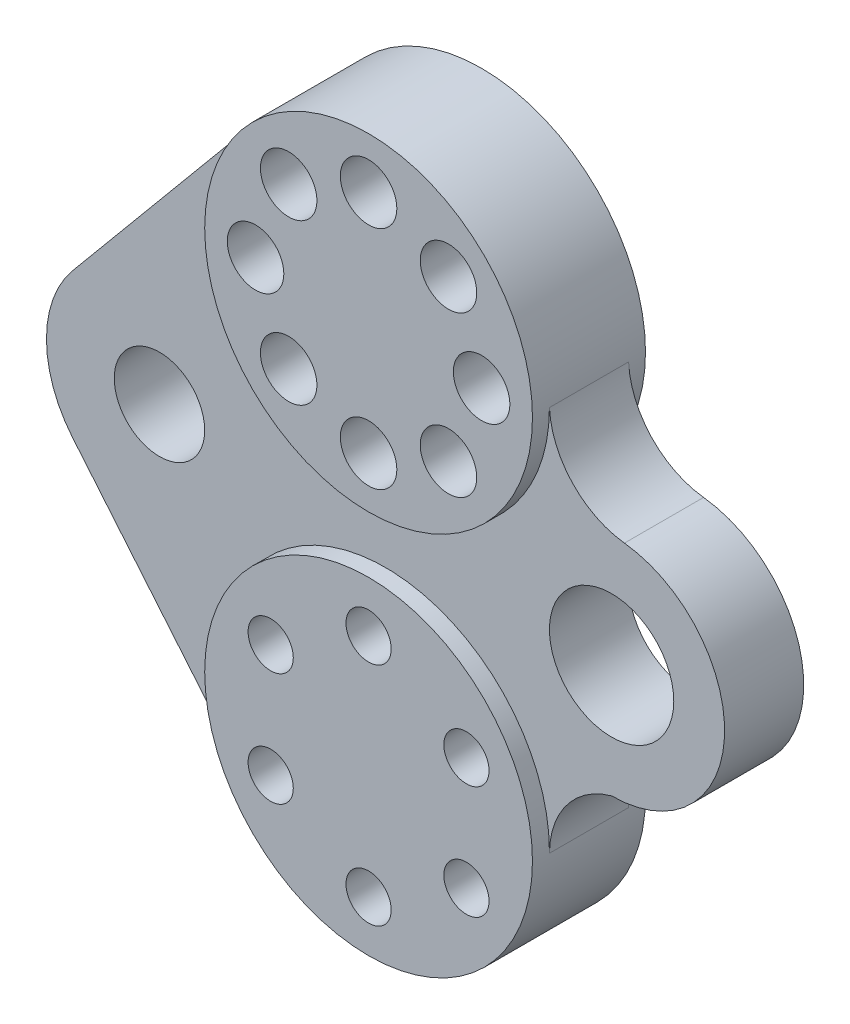
ISO-10303-21;
HEADER;
FILE_DESCRIPTION(('STEP AP214'),'2;1');
FILE_NAME('part.step','',(''),(''),'','','');
FILE_SCHEMA(('AUTOMOTIVE_DESIGN { 1 0 10303 214 1 1 1 1 }'));
ENDSEC;
DATA;
#1=APPLICATION_CONTEXT('core data for automotive mechanical design processes');
#2=APPLICATION_PROTOCOL_DEFINITION('international standard','automotive_design',2000,#1);
#3=PRODUCT_CONTEXT('',#1,'mechanical');
#4=PRODUCT('Part','Part','',(#3));
#5=PRODUCT_RELATED_PRODUCT_CATEGORY('part','',(#4));
#6=PRODUCT_DEFINITION_FORMATION('','',#4);
#7=PRODUCT_DEFINITION_CONTEXT('part definition',#1,'design');
#8=PRODUCT_DEFINITION('design','',#6,#7);
#9=PRODUCT_DEFINITION_SHAPE('','',#8);
#10=(LENGTH_UNIT() NAMED_UNIT(*) SI_UNIT(.MILLI.,.METRE.));
#11=(NAMED_UNIT(*) PLANE_ANGLE_UNIT() SI_UNIT($,.RADIAN.));
#12=(NAMED_UNIT(*) SI_UNIT($,.STERADIAN.) SOLID_ANGLE_UNIT());
#13=UNCERTAINTY_MEASURE_WITH_UNIT(LENGTH_MEASURE(1.E-05),#10,'distance_accuracy_value','');
#14=(GEOMETRIC_REPRESENTATION_CONTEXT(3) GLOBAL_UNCERTAINTY_ASSIGNED_CONTEXT((#13)) GLOBAL_UNIT_ASSIGNED_CONTEXT((#10,
#11,#12)) REPRESENTATION_CONTEXT('',''));
#15=CARTESIAN_POINT('',(0.,0.,0.));
#16=DIRECTION('',(0.,0.,1.));
#17=DIRECTION('',(1.,0.,0.));
#18=AXIS2_PLACEMENT_3D('',#15,#16,#17);
#19=CARTESIAN_POINT('',(0.,20.,10.));
#20=DIRECTION('',(0.,0.,-1.));
#21=DIRECTION('',(-1.,0.,0.));
#22=AXIS2_PLACEMENT_3D('',#19,#20,#21);
#23=CYLINDRICAL_SURFACE('',#22,5.);
#24=CARTESIAN_POINT('',(0.,20.,10.));
#25=DIRECTION('',(0.,0.,1.));
#26=DIRECTION('',(1.,0.,0.));
#27=AXIS2_PLACEMENT_3D('',#24,#25,#26);
#28=CIRCLE('',#27,5.);
#29=CARTESIAN_POINT('',(5.,20.,10.));
#30=VERTEX_POINT('',#29);
#31=EDGE_CURVE('E57',#30,#30,#28,.T.);
#32=ORIENTED_EDGE('',*,*,#31,.T.);
#33=EDGE_LOOP('',(#32));
#34=FACE_BOUND('',#33,.T.);
#35=CARTESIAN_POINT('',(0.,20.,-10.));
#36=DIRECTION('',(0.,0.,1.));
#37=DIRECTION('',(1.,0.,0.));
#38=AXIS2_PLACEMENT_3D('',#35,#36,#37);
#39=CIRCLE('',#38,5.);
#40=CARTESIAN_POINT('',(5.,20.,-10.));
#41=VERTEX_POINT('',#40);
#42=EDGE_CURVE('E213',#41,#41,#39,.T.);
#43=ORIENTED_EDGE('',*,*,#42,.F.);
#44=EDGE_LOOP('',(#43));
#45=FACE_BOUND('',#44,.T.);
#46=ADVANCED_FACE('F50',(#34,#45),#23,.F.);
#47=CARTESIAN_POINT('',(14.142135623731,14.1421356237309,10.));
#48=DIRECTION('',(0.,0.,-1.));
#49=DIRECTION('',(-1.,0.,0.));
#50=AXIS2_PLACEMENT_3D('',#47,#48,#49);
#51=CYLINDRICAL_SURFACE('',#50,5.);
#52=CARTESIAN_POINT('',(14.142135623731,14.1421356237309,10.));
#53=DIRECTION('',(0.,0.,1.));
#54=DIRECTION('',(1.,0.,0.));
#55=AXIS2_PLACEMENT_3D('',#52,#53,#54);
#56=CIRCLE('',#55,5.);
#57=CARTESIAN_POINT('',(19.142135623731,14.1421356237309,10.));
#58=VERTEX_POINT('',#57);
#59=EDGE_CURVE('E186',#58,#58,#56,.T.);
#60=ORIENTED_EDGE('',*,*,#59,.T.);
#61=EDGE_LOOP('',(#60));
#62=FACE_BOUND('',#61,.T.);
#63=CARTESIAN_POINT('',(14.142135623731,14.1421356237309,-10.));
#64=DIRECTION('',(0.,0.,1.));
#65=DIRECTION('',(1.,0.,0.));
#66=AXIS2_PLACEMENT_3D('',#63,#64,#65);
#67=CIRCLE('',#66,5.);
#68=CARTESIAN_POINT('',(19.142135623731,14.1421356237309,-10.));
#69=VERTEX_POINT('',#68);
#70=EDGE_CURVE('E211',#69,#69,#67,.T.);
#71=ORIENTED_EDGE('',*,*,#70,.F.);
#72=EDGE_LOOP('',(#71));
#73=FACE_BOUND('',#72,.T.);
#74=ADVANCED_FACE('F239',(#62,#73),#51,.F.);
#75=CARTESIAN_POINT('',(20.,0.,10.));
#76=DIRECTION('',(0.,0.,-1.));
#77=DIRECTION('',(-1.,0.,0.));
#78=AXIS2_PLACEMENT_3D('',#75,#76,#77);
#79=CYLINDRICAL_SURFACE('',#78,5.);
#80=CARTESIAN_POINT('',(20.,0.,10.));
#81=DIRECTION('',(0.,0.,1.));
#82=DIRECTION('',(1.,0.,0.));
#83=AXIS2_PLACEMENT_3D('',#80,#81,#82);
#84=CIRCLE('',#83,5.);
#85=CARTESIAN_POINT('',(25.,0.,10.));
#86=VERTEX_POINT('',#85);
#87=EDGE_CURVE('E187',#86,#86,#84,.T.);
#88=ORIENTED_EDGE('',*,*,#87,.T.);
#89=EDGE_LOOP('',(#88));
#90=FACE_BOUND('',#89,.T.);
#91=CARTESIAN_POINT('',(20.,0.,-10.));
#92=DIRECTION('',(0.,0.,1.));
#93=DIRECTION('',(1.,0.,0.));
#94=AXIS2_PLACEMENT_3D('',#91,#92,#93);
#95=CIRCLE('',#94,5.);
#96=CARTESIAN_POINT('',(25.,0.,-10.));
#97=VERTEX_POINT('',#96);
#98=EDGE_CURVE('E208',#97,#97,#95,.T.);
#99=ORIENTED_EDGE('',*,*,#98,.F.);
#100=EDGE_LOOP('',(#99));
#101=FACE_BOUND('',#100,.T.);
#102=ADVANCED_FACE('F243',(#90,#101),#79,.F.);
#103=CARTESIAN_POINT('',(14.1421356237305,-14.1421356237305,10.));
#104=DIRECTION('',(0.,0.,-1.));
#105=DIRECTION('',(-1.,0.,0.));
#106=AXIS2_PLACEMENT_3D('',#103,#104,#105);
#107=CYLINDRICAL_SURFACE('',#106,5.00000000000027);
#108=CARTESIAN_POINT('',(14.1421356237305,-14.1421356237305,10.));
#109=DIRECTION('',(0.,0.,1.));
#110=DIRECTION('',(1.,0.,0.));
#111=AXIS2_PLACEMENT_3D('',#108,#109,#110);
#112=CIRCLE('',#111,5.00000000000027);
#113=CARTESIAN_POINT('',(19.1421356237308,-14.1421356237305,10.));
#114=VERTEX_POINT('',#113);
#115=EDGE_CURVE('E181',#114,#114,#112,.T.);
#116=ORIENTED_EDGE('',*,*,#115,.T.);
#117=EDGE_LOOP('',(#116));
#118=FACE_BOUND('',#117,.T.);
#119=CARTESIAN_POINT('',(14.1421356237305,-14.1421356237305,-10.));
#120=DIRECTION('',(0.,0.,1.));
#121=DIRECTION('',(1.,0.,0.));
#122=AXIS2_PLACEMENT_3D('',#119,#120,#121);
#123=CIRCLE('',#122,5.00000000000027);
#124=CARTESIAN_POINT('',(19.1421356237308,-14.1421356237305,-10.));
#125=VERTEX_POINT('',#124);
#126=EDGE_CURVE('E202',#125,#125,#123,.T.);
#127=ORIENTED_EDGE('',*,*,#126,.F.);
#128=EDGE_LOOP('',(#127));
#129=FACE_BOUND('',#128,.T.);
#130=ADVANCED_FACE('F252',(#118,#129),#107,.F.);
#131=CARTESIAN_POINT('',(-2.39579325769986E-13,-19.9999999999994,10.));
#132=DIRECTION('',(0.,0.,-1.));
#133=DIRECTION('',(-1.,0.,0.));
#134=AXIS2_PLACEMENT_3D('',#131,#132,#133);
#135=CYLINDRICAL_SURFACE('',#134,5.00000000000008);
#136=CARTESIAN_POINT('',(-2.39579325769986E-13,-19.9999999999994,10.));
#137=DIRECTION('',(0.,0.,1.));
#138=DIRECTION('',(1.,0.,0.));
#139=AXIS2_PLACEMENT_3D('',#136,#137,#138);
#140=CIRCLE('',#139,5.00000000000008);
#141=CARTESIAN_POINT('',(4.99999999999984,-19.9999999999994,10.));
#142=VERTEX_POINT('',#141);
#143=EDGE_CURVE('E178',#142,#142,#140,.T.);
#144=ORIENTED_EDGE('',*,*,#143,.T.);
#145=EDGE_LOOP('',(#144));
#146=FACE_BOUND('',#145,.T.);
#147=CARTESIAN_POINT('',(-2.39579325769986E-13,-19.9999999999994,-10.));
#148=DIRECTION('',(0.,0.,1.));
#149=DIRECTION('',(1.,0.,0.));
#150=AXIS2_PLACEMENT_3D('',#147,#148,#149);
#151=CIRCLE('',#150,5.00000000000008);
#152=CARTESIAN_POINT('',(4.99999999999984,-19.9999999999994,-10.));
#153=VERTEX_POINT('',#152);
#154=EDGE_CURVE('E205',#153,#153,#151,.T.);
#155=ORIENTED_EDGE('',*,*,#154,.F.);
#156=EDGE_LOOP('',(#155));
#157=FACE_BOUND('',#156,.T.);
#158=ADVANCED_FACE('F258',(#146,#157),#135,.F.);
#159=CARTESIAN_POINT('',(-14.1421356237309,-14.1421356237304,10.));
#160=DIRECTION('',(0.,0.,-1.));
#161=DIRECTION('',(-1.,0.,0.));
#162=AXIS2_PLACEMENT_3D('',#159,#160,#161);
#163=CYLINDRICAL_SURFACE('',#162,4.9999999999999);
#164=CARTESIAN_POINT('',(-14.1421356237309,-14.1421356237304,10.));
#165=DIRECTION('',(0.,0.,1.));
#166=DIRECTION('',(1.,0.,0.));
#167=AXIS2_PLACEMENT_3D('',#164,#165,#166);
#168=CIRCLE('',#167,4.9999999999999);
#169=CARTESIAN_POINT('',(-9.14213562373105,-14.1421356237304,10.));
#170=VERTEX_POINT('',#169);
#171=EDGE_CURVE('E179',#170,#170,#168,.T.);
#172=ORIENTED_EDGE('',*,*,#171,.T.);
#173=EDGE_LOOP('',(#172));
#174=FACE_BOUND('',#173,.T.);
#175=CARTESIAN_POINT('',(-14.1421356237309,-14.1421356237304,-10.));
#176=DIRECTION('',(0.,0.,1.));
#177=DIRECTION('',(1.,0.,0.));
#178=AXIS2_PLACEMENT_3D('',#175,#176,#177);
#179=CIRCLE('',#178,4.9999999999999);
#180=CARTESIAN_POINT('',(-9.14213562373105,-14.1421356237304,-10.));
#181=VERTEX_POINT('',#180);
#182=EDGE_CURVE('E200',#181,#181,#179,.T.);
#183=ORIENTED_EDGE('',*,*,#182,.F.);
#184=EDGE_LOOP('',(#183));
#185=FACE_BOUND('',#184,.T.);
#186=ADVANCED_FACE('F257',(#174,#185),#163,.F.);
#187=CARTESIAN_POINT('',(-20.,2.09488880330588E-13,10.));
#188=DIRECTION('',(0.,0.,-1.));
#189=DIRECTION('',(-1.,0.,0.));
#190=AXIS2_PLACEMENT_3D('',#187,#188,#189);
#191=CYLINDRICAL_SURFACE('',#190,5.);
#192=CARTESIAN_POINT('',(-20.,2.09488880330588E-13,10.));
#193=DIRECTION('',(0.,0.,1.));
#194=DIRECTION('',(1.,0.,0.));
#195=AXIS2_PLACEMENT_3D('',#192,#193,#194);
#196=CIRCLE('',#195,5.);
#197=CARTESIAN_POINT('',(-15.,2.09488880330588E-13,10.));
#198=VERTEX_POINT('',#197);
#199=EDGE_CURVE('E171',#198,#198,#196,.T.);
#200=ORIENTED_EDGE('',*,*,#199,.T.);
#201=EDGE_LOOP('',(#200));
#202=FACE_BOUND('',#201,.T.);
#203=CARTESIAN_POINT('',(-20.,2.09488880330588E-13,-10.));
#204=DIRECTION('',(0.,0.,1.));
#205=DIRECTION('',(1.,0.,0.));
#206=AXIS2_PLACEMENT_3D('',#203,#204,#205);
#207=CIRCLE('',#206,5.);
#208=CARTESIAN_POINT('',(-15.,2.09488880330588E-13,-10.));
#209=VERTEX_POINT('',#208);
#210=EDGE_CURVE('E198',#209,#209,#207,.T.);
#211=ORIENTED_EDGE('',*,*,#210,.F.);
#212=EDGE_LOOP('',(#211));
#213=FACE_BOUND('',#212,.T.);
#214=ADVANCED_FACE('F263',(#202,#213),#191,.F.);
#215=CARTESIAN_POINT('',(-14.1421356237308,14.1421356237311,10.));
#216=DIRECTION('',(0.,0.,-1.));
#217=DIRECTION('',(-1.,0.,0.));
#218=AXIS2_PLACEMENT_3D('',#215,#216,#217);
#219=CYLINDRICAL_SURFACE('',#218,5.);
#220=CARTESIAN_POINT('',(-14.1421356237308,14.1421356237311,10.));
#221=DIRECTION('',(0.,0.,1.));
#222=DIRECTION('',(1.,0.,0.));
#223=AXIS2_PLACEMENT_3D('',#220,#221,#222);
#224=CIRCLE('',#223,5.);
#225=CARTESIAN_POINT('',(-9.14213562373078,14.1421356237311,10.));
#226=VERTEX_POINT('',#225);
#227=EDGE_CURVE('E172',#226,#226,#224,.T.);
#228=ORIENTED_EDGE('',*,*,#227,.T.);
#229=EDGE_LOOP('',(#228));
#230=FACE_BOUND('',#229,.T.);
#231=CARTESIAN_POINT('',(-14.1421356237308,14.1421356237311,-10.));
#232=DIRECTION('',(0.,0.,1.));
#233=DIRECTION('',(1.,0.,0.));
#234=AXIS2_PLACEMENT_3D('',#231,#232,#233);
#235=CIRCLE('',#234,5.);
#236=CARTESIAN_POINT('',(-9.14213562373078,14.1421356237311,-10.));
#237=VERTEX_POINT('',#236);
#238=EDGE_CURVE('E135',#237,#237,#235,.T.);
#239=ORIENTED_EDGE('',*,*,#238,.F.);
#240=EDGE_LOOP('',(#239));
#241=FACE_BOUND('',#240,.T.);
#242=ADVANCED_FACE('F47',(#230,#241),#219,.F.);
#243=CARTESIAN_POINT('',(0.,0.,10.));
#244=DIRECTION('',(0.,0.,-1.));
#245=DIRECTION('',(-1.,0.,0.));
#246=AXIS2_PLACEMENT_3D('',#243,#244,#245);
#247=CYLINDRICAL_SURFACE('',#246,29.);
#248=DIRECTION('',(0.,0.,-1.));
#249=VECTOR('',#248,1.);
#250=CARTESIAN_POINT('',(-22.291841993341,18.5492258745188,7.));
#251=LINE('',#250,#249);
#252=CARTESIAN_POINT('',(-22.291841993341,18.5492258745188,7.));
#253=VERTEX_POINT('',#252);
#254=CARTESIAN_POINT('',(-22.291841993341,18.5492258745188,-7.));
#255=VERTEX_POINT('',#254);
#256=EDGE_CURVE('E66',#253,#255,#251,.T.);
#257=ORIENTED_EDGE('',*,*,#256,.F.);
#258=CARTESIAN_POINT('',(0.,0.,7.));
#259=DIRECTION('',(0.,0.,1.));
#260=DIRECTION('',(1.,0.,0.));
#261=AXIS2_PLACEMENT_3D('',#258,#259,#260);
#262=CIRCLE('',#261,29.);
#263=CARTESIAN_POINT('',(29.,0.,7.));
#264=VERTEX_POINT('',#263);
#265=EDGE_CURVE('E61',#253,#264,#262,.T.);
#266=ORIENTED_EDGE('',*,*,#265,.T.);
#267=DIRECTION('',(0.,0.,-1.));
#268=VECTOR('',#267,1.);
#269=CARTESIAN_POINT('',(29.,0.,7.));
#270=LINE('',#269,#268);
#271=CARTESIAN_POINT('',(29.,0.,-7.));
#272=VERTEX_POINT('',#271);
#273=EDGE_CURVE('E167',#264,#272,#270,.T.);
#274=ORIENTED_EDGE('',*,*,#273,.T.);
#275=CARTESIAN_POINT('',(0.,0.,-7.));
#276=DIRECTION('',(0.,0.,1.));
#277=DIRECTION('',(1.,0.,0.));
#278=AXIS2_PLACEMENT_3D('',#275,#276,#277);
#279=CIRCLE('',#278,29.);
#280=EDGE_CURVE('E148',#255,#272,#279,.T.);
#281=ORIENTED_EDGE('',*,*,#280,.F.);
#282=EDGE_LOOP('',(#257,#266,#274,#281));
#283=FACE_BOUND('',#282,.T.);
#284=CARTESIAN_POINT('',(0.,0.,10.));
#285=DIRECTION('',(0.,0.,1.));
#286=DIRECTION('',(1.,0.,0.));
#287=AXIS2_PLACEMENT_3D('',#284,#285,#286);
#288=CIRCLE('',#287,29.);
#289=CARTESIAN_POINT('',(29.,0.,10.));
#290=VERTEX_POINT('',#289);
#291=EDGE_CURVE('E11',#290,#290,#288,.T.);
#292=ORIENTED_EDGE('',*,*,#291,.F.);
#293=EDGE_LOOP('',(#292));
#294=FACE_BOUND('',#293,.T.);
#295=CARTESIAN_POINT('',(0.,0.,-10.));
#296=DIRECTION('',(0.,0.,1.));
#297=DIRECTION('',(1.,0.,0.));
#298=AXIS2_PLACEMENT_3D('',#295,#296,#297);
#299=CIRCLE('',#298,29.);
#300=CARTESIAN_POINT('',(29.,0.,-10.));
#301=VERTEX_POINT('',#300);
#302=EDGE_CURVE('E51',#301,#301,#299,.T.);
#303=ORIENTED_EDGE('',*,*,#302,.T.);
#304=EDGE_LOOP('',(#303));
#305=FACE_BOUND('',#304,.T.);
#306=ADVANCED_FACE('F219',(#283,#294,#305),#247,.T.);
#307=CARTESIAN_POINT('',(0.,0.,10.));
#308=DIRECTION('',(0.,0.,1.));
#309=DIRECTION('',(1.,0.,0.));
#310=AXIS2_PLACEMENT_3D('',#307,#308,#309);
#311=PLANE('',#310);
#312=ORIENTED_EDGE('',*,*,#227,.F.);
#313=EDGE_LOOP('',(#312));
#314=FACE_BOUND('',#313,.T.);
#315=ORIENTED_EDGE('',*,*,#199,.F.);
#316=EDGE_LOOP('',(#315));
#317=FACE_BOUND('',#316,.T.);
#318=ORIENTED_EDGE('',*,*,#171,.F.);
#319=EDGE_LOOP('',(#318));
#320=FACE_BOUND('',#319,.T.);
#321=ORIENTED_EDGE('',*,*,#143,.F.);
#322=EDGE_LOOP('',(#321));
#323=FACE_BOUND('',#322,.T.);
#324=ORIENTED_EDGE('',*,*,#115,.F.);
#325=EDGE_LOOP('',(#324));
#326=FACE_BOUND('',#325,.T.);
#327=ORIENTED_EDGE('',*,*,#87,.F.);
#328=EDGE_LOOP('',(#327));
#329=FACE_BOUND('',#328,.T.);
#330=ORIENTED_EDGE('',*,*,#59,.F.);
#331=EDGE_LOOP('',(#330));
#332=FACE_BOUND('',#331,.T.);
#333=ORIENTED_EDGE('',*,*,#31,.F.);
#334=EDGE_LOOP('',(#333));
#335=FACE_BOUND('',#334,.T.);
#336=ORIENTED_EDGE('',*,*,#291,.T.);
#337=EDGE_LOOP('',(#336));
#338=FACE_BOUND('',#337,.T.);
#339=ADVANCED_FACE('F221',(#314,#317,#320,#323,#326,#329,#332,#335,#338),#311,.T.);
#340=CARTESIAN_POINT('',(0.,0.,-10.));
#341=DIRECTION('',(0.,0.,1.));
#342=DIRECTION('',(1.,0.,0.));
#343=AXIS2_PLACEMENT_3D('',#340,#341,#342);
#344=PLANE('',#343);
#345=ORIENTED_EDGE('',*,*,#238,.T.);
#346=EDGE_LOOP('',(#345));
#347=FACE_BOUND('',#346,.T.);
#348=ORIENTED_EDGE('',*,*,#210,.T.);
#349=EDGE_LOOP('',(#348));
#350=FACE_BOUND('',#349,.T.);
#351=ORIENTED_EDGE('',*,*,#182,.T.);
#352=EDGE_LOOP('',(#351));
#353=FACE_BOUND('',#352,.T.);
#354=ORIENTED_EDGE('',*,*,#154,.T.);
#355=EDGE_LOOP('',(#354));
#356=FACE_BOUND('',#355,.T.);
#357=ORIENTED_EDGE('',*,*,#126,.T.);
#358=EDGE_LOOP('',(#357));
#359=FACE_BOUND('',#358,.T.);
#360=ORIENTED_EDGE('',*,*,#98,.T.);
#361=EDGE_LOOP('',(#360));
#362=FACE_BOUND('',#361,.T.);
#363=ORIENTED_EDGE('',*,*,#70,.T.);
#364=EDGE_LOOP('',(#363));
#365=FACE_BOUND('',#364,.T.);
#366=ORIENTED_EDGE('',*,*,#42,.T.);
#367=EDGE_LOOP('',(#366));
#368=FACE_BOUND('',#367,.T.);
#369=ORIENTED_EDGE('',*,*,#302,.F.);
#370=EDGE_LOOP('',(#369));
#371=FACE_BOUND('',#370,.T.);
#372=ADVANCED_FACE('F225',(#347,#350,#353,#356,#359,#362,#365,#368,#371),#344,.F.);
#373=CARTESIAN_POINT('',(43.9976215578597,-68.4574901653135,7.));
#374=DIRECTION('',(0.,0.,-1.));
#375=DIRECTION('',(-1.,0.,0.));
#376=AXIS2_PLACEMENT_3D('',#373,#374,#375);
#377=CYLINDRICAL_SURFACE('',#376,15.);
#378=CARTESIAN_POINT('',(43.9976215578597,-68.4574901653135,-7.));
#379=DIRECTION('',(0.,0.,1.));
#380=DIRECTION('',(1.,0.,0.));
#381=AXIS2_PLACEMENT_3D('',#378,#379,#380);
#382=CIRCLE('',#381,15.);
#383=CARTESIAN_POINT('',(28.9984323904075,-68.3015276089566,-7.));
#384=VERTEX_POINT('',#383);
#385=CARTESIAN_POINT('',(40.,-54.,-7.));
#386=VERTEX_POINT('',#385);
#387=EDGE_CURVE('E124',#384,#386,#382,.F.);
#388=ORIENTED_EDGE('',*,*,#387,.T.);
#389=DIRECTION('',(0.,0.,-1.));
#390=VECTOR('',#389,1.);
#391=CARTESIAN_POINT('',(40.,-54.,7.));
#392=LINE('',#391,#390);
#393=CARTESIAN_POINT('',(40.,-54.,7.));
#394=VERTEX_POINT('',#393);
#395=EDGE_CURVE('E134',#394,#386,#392,.T.);
#396=ORIENTED_EDGE('',*,*,#395,.F.);
#397=CARTESIAN_POINT('',(43.9976215578597,-68.4574901653135,7.));
#398=DIRECTION('',(0.,0.,1.));
#399=DIRECTION('',(1.,0.,0.));
#400=AXIS2_PLACEMENT_3D('',#397,#398,#399);
#401=CIRCLE('',#400,15.);
#402=CARTESIAN_POINT('',(28.9984323904075,-68.3015276089566,7.));
#403=VERTEX_POINT('',#402);
#404=EDGE_CURVE('E128',#403,#394,#401,.F.);
#405=ORIENTED_EDGE('',*,*,#404,.F.);
#406=DIRECTION('',(0.,0.,-1.));
#407=VECTOR('',#406,1.);
#408=CARTESIAN_POINT('',(28.9984323904075,-68.3015276089566,7.));
#409=LINE('',#408,#407);
#410=EDGE_CURVE('E113',#403,#384,#409,.T.);
#411=ORIENTED_EDGE('',*,*,#410,.T.);
#412=EDGE_LOOP('',(#388,#396,#405,#411));
#413=FACE_BOUND('',#412,.T.);
#414=ADVANCED_FACE('F130',(#413),#377,.F.);
#415=CARTESIAN_POINT('',(40.,-34.,7.));
#416=DIRECTION('',(0.,0.,-1.));
#417=DIRECTION('',(-1.,0.,0.));
#418=AXIS2_PLACEMENT_3D('',#415,#416,#417);
#419=CYLINDRICAL_SURFACE('',#418,20.);
#420=CARTESIAN_POINT('',(40.,-34.,-7.));
#421=DIRECTION('',(0.,0.,1.));
#422=DIRECTION('',(1.,0.,0.));
#423=AXIS2_PLACEMENT_3D('',#420,#421,#422);
#424=CIRCLE('',#423,20.);
#425=CARTESIAN_POINT('',(42.2743262718756,-14.1297347775865,-7.));
#426=VERTEX_POINT('',#425);
#427=EDGE_CURVE('E140',#386,#426,#424,.T.);
#428=ORIENTED_EDGE('',*,*,#427,.T.);
#429=DIRECTION('',(0.,0.,-1.));
#430=VECTOR('',#429,1.);
#431=CARTESIAN_POINT('',(42.2743262718756,-14.1297347775865,7.));
#432=LINE('',#431,#430);
#433=CARTESIAN_POINT('',(42.2743262718756,-14.1297347775865,7.));
#434=VERTEX_POINT('',#433);
#435=EDGE_CURVE('E169',#434,#426,#432,.T.);
#436=ORIENTED_EDGE('',*,*,#435,.F.);
#437=CARTESIAN_POINT('',(40.,-34.,7.));
#438=DIRECTION('',(0.,0.,1.));
#439=DIRECTION('',(1.,0.,0.));
#440=AXIS2_PLACEMENT_3D('',#437,#438,#439);
#441=CIRCLE('',#440,20.);
#442=EDGE_CURVE('E689',#394,#434,#441,.T.);
#443=ORIENTED_EDGE('',*,*,#442,.F.);
#444=ORIENTED_EDGE('',*,*,#395,.T.);
#445=EDGE_LOOP('',(#428,#436,#443,#444));
#446=FACE_BOUND('',#445,.T.);
#447=ADVANCED_FACE('F234',(#446),#419,.T.);
#448=CARTESIAN_POINT('',(43.9800709757823,0.772964139223671,7.));
#449=DIRECTION('',(0.,0.,-1.));
#450=DIRECTION('',(-1.,0.,0.));
#451=AXIS2_PLACEMENT_3D('',#448,#449,#450);
#452=CYLINDRICAL_SURFACE('',#451,15.);
#453=CARTESIAN_POINT('',(43.9800709757823,0.772964139223671,-7.));
#454=DIRECTION('',(0.,0.,1.));
#455=DIRECTION('',(1.,0.,0.));
#456=AXIS2_PLACEMENT_3D('',#453,#454,#455);
#457=CIRCLE('',#456,15.);
#458=EDGE_CURVE('E143',#272,#426,#457,.T.);
#459=ORIENTED_EDGE('',*,*,#458,.F.);
#460=ORIENTED_EDGE('',*,*,#273,.F.);
#461=CARTESIAN_POINT('',(43.9800709757823,0.772964139223671,7.));
#462=DIRECTION('',(0.,0.,1.));
#463=DIRECTION('',(1.,0.,0.));
#464=AXIS2_PLACEMENT_3D('',#461,#462,#463);
#465=CIRCLE('',#464,15.);
#466=EDGE_CURVE('E686',#264,#434,#465,.T.);
#467=ORIENTED_EDGE('',*,*,#466,.T.);
#468=ORIENTED_EDGE('',*,*,#435,.T.);
#469=EDGE_LOOP('',(#459,#460,#467,#468));
#470=FACE_BOUND('',#469,.T.);
#471=ADVANCED_FACE('F325',(#470),#452,.F.);
#472=CARTESIAN_POINT('',(-22.291841993341,18.5492258745188,7.));
#473=DIRECTION('',(-0.768684206666931,0.639628478431683,0.));
#474=DIRECTION('',(-0.639628478431683,-0.768684206666931,0.));
#475=AXIS2_PLACEMENT_3D('',#472,#473,#474);
#476=PLANE('',#475);
#477=DIRECTION('',(0.639628478431684,0.768684206666931,0.));
#478=VECTOR('',#477,1.);
#479=CARTESIAN_POINT('',(-22.291841993341,18.5492258745188,-7.));
#480=LINE('',#479,#478);
#481=CARTESIAN_POINT('',(-55.3736841333386,-21.2074304313663,-7.));
#482=VERTEX_POINT('',#481);
#483=EDGE_CURVE('E149',#482,#255,#480,.T.);
#484=ORIENTED_EDGE('',*,*,#483,.F.);
#485=DIRECTION('',(0.,0.,-1.));
#486=VECTOR('',#485,1.);
#487=CARTESIAN_POINT('',(-55.3736841333386,-21.2074304313663,7.));
#488=LINE('',#487,#486);
#489=CARTESIAN_POINT('',(-55.3736841333386,-21.2074304313663,7.));
#490=VERTEX_POINT('',#489);
#491=EDGE_CURVE('E162',#490,#482,#488,.T.);
#492=ORIENTED_EDGE('',*,*,#491,.F.);
#493=DIRECTION('',(0.639628478431684,0.768684206666931,0.));
#494=VECTOR('',#493,1.);
#495=CARTESIAN_POINT('',(-22.291841993341,18.5492258745188,7.));
#496=LINE('',#495,#494);
#497=EDGE_CURVE('E691',#490,#253,#496,.T.);
#498=ORIENTED_EDGE('',*,*,#497,.T.);
#499=ORIENTED_EDGE('',*,*,#256,.T.);
#500=EDGE_LOOP('',(#484,#492,#498,#499));
#501=FACE_BOUND('',#500,.T.);
#502=ADVANCED_FACE('F332',(#501),#476,.T.);
#503=CARTESIAN_POINT('',(-40.,-34.,7.));
#504=DIRECTION('',(0.,0.,-1.));
#505=DIRECTION('',(-1.,0.,0.));
#506=AXIS2_PLACEMENT_3D('',#503,#504,#505);
#507=CYLINDRICAL_SURFACE('',#506,20.);
#508=CARTESIAN_POINT('',(-40.,-34.,-7.));
#509=DIRECTION('',(0.,0.,1.));
#510=DIRECTION('',(1.,0.,0.));
#511=AXIS2_PLACEMENT_3D('',#508,#509,#510);
#512=CIRCLE('',#511,20.);
#513=CARTESIAN_POINT('',(-55.3736841333386,-46.7925695686337,-7.));
#514=VERTEX_POINT('',#513);
#515=EDGE_CURVE('E155',#482,#514,#512,.T.);
#516=ORIENTED_EDGE('',*,*,#515,.T.);
#517=DIRECTION('',(0.,0.,-1.));
#518=VECTOR('',#517,1.);
#519=CARTESIAN_POINT('',(-55.3736841333386,-46.7925695686337,7.));
#520=LINE('',#519,#518);
#521=CARTESIAN_POINT('',(-55.3736841333386,-46.7925695686337,7.));
#522=VERTEX_POINT('',#521);
#523=EDGE_CURVE('E157',#522,#514,#520,.T.);
#524=ORIENTED_EDGE('',*,*,#523,.F.);
#525=CARTESIAN_POINT('',(-40.,-34.,7.));
#526=DIRECTION('',(0.,0.,1.));
#527=DIRECTION('',(1.,0.,0.));
#528=AXIS2_PLACEMENT_3D('',#525,#526,#527);
#529=CIRCLE('',#528,20.);
#530=EDGE_CURVE('E698',#490,#522,#529,.T.);
#531=ORIENTED_EDGE('',*,*,#530,.F.);
#532=ORIENTED_EDGE('',*,*,#491,.T.);
#533=EDGE_LOOP('',(#516,#524,#531,#532));
#534=FACE_BOUND('',#533,.T.);
#535=ADVANCED_FACE('F338',(#534),#507,.T.);
#536=CARTESIAN_POINT('',(-40.,-34.,7.));
#537=DIRECTION('',(0.,0.,-1.));
#538=DIRECTION('',(-1.,0.,0.));
#539=AXIS2_PLACEMENT_3D('',#536,#537,#538);
#540=CYLINDRICAL_SURFACE('',#539,8.);
#541=CARTESIAN_POINT('',(-40.,-34.,7.));
#542=DIRECTION('',(0.,0.,1.));
#543=DIRECTION('',(1.,0.,0.));
#544=AXIS2_PLACEMENT_3D('',#541,#542,#543);
#545=CIRCLE('',#544,8.);
#546=CARTESIAN_POINT('',(-32.,-34.,7.));
#547=VERTEX_POINT('',#546);
#548=EDGE_CURVE('E682',#547,#547,#545,.T.);
#549=ORIENTED_EDGE('',*,*,#548,.T.);
#550=EDGE_LOOP('',(#549));
#551=FACE_BOUND('',#550,.T.);
#552=CARTESIAN_POINT('',(-40.,-34.,-7.));
#553=DIRECTION('',(0.,0.,1.));
#554=DIRECTION('',(1.,0.,0.));
#555=AXIS2_PLACEMENT_3D('',#552,#553,#554);
#556=CIRCLE('',#555,8.);
#557=CARTESIAN_POINT('',(-32.,-34.,-7.));
#558=VERTEX_POINT('',#557);
#559=EDGE_CURVE('E125',#558,#558,#556,.T.);
#560=ORIENTED_EDGE('',*,*,#559,.F.);
#561=EDGE_LOOP('',(#560));
#562=FACE_BOUND('',#561,.T.);
#563=ADVANCED_FACE('F349',(#551,#562),#540,.F.);
#564=CARTESIAN_POINT('',(40.,-34.,7.));
#565=DIRECTION('',(0.,0.,-1.));
#566=DIRECTION('',(-1.,0.,0.));
#567=AXIS2_PLACEMENT_3D('',#564,#565,#566);
#568=CYLINDRICAL_SURFACE('',#567,11.);
#569=CARTESIAN_POINT('',(40.,-34.,7.));
#570=DIRECTION('',(0.,0.,1.));
#571=DIRECTION('',(1.,0.,0.));
#572=AXIS2_PLACEMENT_3D('',#569,#570,#571);
#573=CIRCLE('',#572,11.);
#574=CARTESIAN_POINT('',(51.,-34.,7.));
#575=VERTEX_POINT('',#574);
#576=EDGE_CURVE('E160',#575,#575,#573,.T.);
#577=ORIENTED_EDGE('',*,*,#576,.T.);
#578=EDGE_LOOP('',(#577));
#579=FACE_BOUND('',#578,.T.);
#580=CARTESIAN_POINT('',(40.,-34.,-7.));
#581=DIRECTION('',(0.,0.,1.));
#582=DIRECTION('',(1.,0.,0.));
#583=AXIS2_PLACEMENT_3D('',#580,#581,#582);
#584=CIRCLE('',#583,11.);
#585=CARTESIAN_POINT('',(51.,-34.,-7.));
#586=VERTEX_POINT('',#585);
#587=EDGE_CURVE('E701',#586,#586,#584,.T.);
#588=ORIENTED_EDGE('',*,*,#587,.F.);
#589=EDGE_LOOP('',(#588));
#590=FACE_BOUND('',#589,.T.);
#591=ADVANCED_FACE('F358',(#579,#590),#568,.F.);
#592=CARTESIAN_POINT('',(-55.7255590396698,-46.3696980231353,7.));
#593=DIRECTION('',(0.768684206666931,0.639628478431683,0.));
#594=DIRECTION('',(-0.639628478431683,0.768684206666931,0.));
#595=AXIS2_PLACEMENT_3D('',#592,#593,#594);
#596=PLANE('',#595);
#597=DIRECTION('',(0.639628478431684,-0.768684206666931,0.));
#598=VECTOR('',#597,1.);
#599=CARTESIAN_POINT('',(-55.7255590396698,-46.3696980231353,-7.));
#600=LINE('',#599,#598);
#601=CARTESIAN_POINT('',(-22.291841993341,-86.5492258745188,-7.));
#602=VERTEX_POINT('',#601);
#603=EDGE_CURVE('E154',#514,#602,#600,.T.);
#604=ORIENTED_EDGE('',*,*,#603,.T.);
#605=DIRECTION('',(0.,0.,-1.));
#606=VECTOR('',#605,1.);
#607=CARTESIAN_POINT('',(-22.291841993341,-86.5492258745188,7.));
#608=LINE('',#607,#606);
#609=CARTESIAN_POINT('',(-22.291841993341,-86.5492258745188,7.));
#610=VERTEX_POINT('',#609);
#611=EDGE_CURVE('E119',#610,#602,#608,.T.);
#612=ORIENTED_EDGE('',*,*,#611,.F.);
#613=DIRECTION('',(0.639628478431684,-0.768684206666931,0.));
#614=VECTOR('',#613,1.);
#615=CARTESIAN_POINT('',(-55.7255590396698,-46.3696980231353,7.));
#616=LINE('',#615,#614);
#617=EDGE_CURVE('E159',#522,#610,#616,.T.);
#618=ORIENTED_EDGE('',*,*,#617,.F.);
#619=ORIENTED_EDGE('',*,*,#523,.T.);
#620=EDGE_LOOP('',(#604,#612,#618,#619));
#621=FACE_BOUND('',#620,.T.);
#622=ADVANCED_FACE('F372',(#621),#596,.F.);
#623=CARTESIAN_POINT('',(0.,0.,7.));
#624=DIRECTION('',(0.,0.,1.));
#625=DIRECTION('',(1.,0.,0.));
#626=AXIS2_PLACEMENT_3D('',#623,#624,#625);
#627=PLANE('',#626);
#628=ORIENTED_EDGE('',*,*,#576,.F.);
#629=EDGE_LOOP('',(#628));
#630=FACE_BOUND('',#629,.T.);
#631=ORIENTED_EDGE('',*,*,#548,.F.);
#632=EDGE_LOOP('',(#631));
#633=FACE_BOUND('',#632,.T.);
#634=CARTESIAN_POINT('',(0.,-68.,7.));
#635=DIRECTION('',(0.,0.,1.));
#636=DIRECTION('',(1.,0.,0.));
#637=AXIS2_PLACEMENT_3D('',#634,#635,#636);
#638=CIRCLE('',#637,29.);
#639=EDGE_CURVE('E681',#403,#610,#638,.T.);
#640=ORIENTED_EDGE('',*,*,#639,.F.);
#641=ORIENTED_EDGE('',*,*,#404,.T.);
#642=ORIENTED_EDGE('',*,*,#442,.T.);
#643=ORIENTED_EDGE('',*,*,#466,.F.);
#644=ORIENTED_EDGE('',*,*,#265,.F.);
#645=ORIENTED_EDGE('',*,*,#497,.F.);
#646=ORIENTED_EDGE('',*,*,#530,.T.);
#647=ORIENTED_EDGE('',*,*,#617,.T.);
#648=EDGE_LOOP('',(#640,#641,#642,#643,#644,#645,#646,#647));
#649=FACE_BOUND('',#648,.T.);
#650=ADVANCED_FACE('F387',(#630,#633,#649),#627,.T.);
#651=CARTESIAN_POINT('',(0.,0.,-7.));
#652=DIRECTION('',(0.,0.,1.));
#653=DIRECTION('',(1.,0.,0.));
#654=AXIS2_PLACEMENT_3D('',#651,#652,#653);
#655=PLANE('',#654);
#656=ORIENTED_EDGE('',*,*,#587,.T.);
#657=EDGE_LOOP('',(#656));
#658=FACE_BOUND('',#657,.T.);
#659=ORIENTED_EDGE('',*,*,#559,.T.);
#660=EDGE_LOOP('',(#659));
#661=FACE_BOUND('',#660,.T.);
#662=CARTESIAN_POINT('',(0.,-68.,-7.));
#663=DIRECTION('',(0.,0.,1.));
#664=DIRECTION('',(1.,0.,0.));
#665=AXIS2_PLACEMENT_3D('',#662,#663,#664);
#666=CIRCLE('',#665,29.);
#667=EDGE_CURVE('E112',#384,#602,#666,.T.);
#668=ORIENTED_EDGE('',*,*,#667,.T.);
#669=ORIENTED_EDGE('',*,*,#603,.F.);
#670=ORIENTED_EDGE('',*,*,#515,.F.);
#671=ORIENTED_EDGE('',*,*,#483,.T.);
#672=ORIENTED_EDGE('',*,*,#280,.T.);
#673=ORIENTED_EDGE('',*,*,#458,.T.);
#674=ORIENTED_EDGE('',*,*,#427,.F.);
#675=ORIENTED_EDGE('',*,*,#387,.F.);
#676=EDGE_LOOP('',(#668,#669,#670,#671,#672,#673,#674,#675));
#677=FACE_BOUND('',#676,.T.);
#678=ADVANCED_FACE('F133',(#658,#661,#677),#655,.F.);
#679=CARTESIAN_POINT('',(0.,-88.,10.));
#680=DIRECTION('',(0.,0.,-1.));
#681=DIRECTION('',(-1.,0.,0.));
#682=AXIS2_PLACEMENT_3D('',#679,#680,#681);
#683=CYLINDRICAL_SURFACE('',#682,4.);
#684=CARTESIAN_POINT('',(0.,-88.,10.));
#685=DIRECTION('',(0.,0.,1.));
#686=DIRECTION('',(1.,0.,0.));
#687=AXIS2_PLACEMENT_3D('',#684,#685,#686);
#688=CIRCLE('',#687,4.);
#689=CARTESIAN_POINT('',(4.,-88.,10.));
#690=VERTEX_POINT('',#689);
#691=EDGE_CURVE('E709',#690,#690,#688,.T.);
#692=ORIENTED_EDGE('',*,*,#691,.T.);
#693=EDGE_LOOP('',(#692));
#694=FACE_BOUND('',#693,.T.);
#695=CARTESIAN_POINT('',(0.,-88.,-10.));
#696=DIRECTION('',(0.,0.,1.));
#697=DIRECTION('',(1.,0.,0.));
#698=AXIS2_PLACEMENT_3D('',#695,#696,#697);
#699=CIRCLE('',#698,4.);
#700=CARTESIAN_POINT('',(4.,-88.,-10.));
#701=VERTEX_POINT('',#700);
#702=EDGE_CURVE('E667',#701,#701,#699,.T.);
#703=ORIENTED_EDGE('',*,*,#702,.F.);
#704=EDGE_LOOP('',(#703));
#705=FACE_BOUND('',#704,.T.);
#706=ADVANCED_FACE('F401',(#694,#705),#683,.F.);
#707=CARTESIAN_POINT('',(-17.3205080756888,-78.,10.));
#708=DIRECTION('',(0.,0.,-1.));
#709=DIRECTION('',(-1.,0.,0.));
#710=AXIS2_PLACEMENT_3D('',#707,#708,#709);
#711=CYLINDRICAL_SURFACE('',#710,4.00000000000001);
#712=CARTESIAN_POINT('',(-17.3205080756888,-78.,10.));
#713=DIRECTION('',(0.,0.,1.));
#714=DIRECTION('',(1.,0.,0.));
#715=AXIS2_PLACEMENT_3D('',#712,#713,#714);
#716=CIRCLE('',#715,4.00000000000001);
#717=CARTESIAN_POINT('',(-13.3205080756888,-78.,10.));
#718=VERTEX_POINT('',#717);
#719=EDGE_CURVE('E714',#718,#718,#716,.T.);
#720=ORIENTED_EDGE('',*,*,#719,.T.);
#721=EDGE_LOOP('',(#720));
#722=FACE_BOUND('',#721,.T.);
#723=CARTESIAN_POINT('',(-17.3205080756888,-78.,-10.));
#724=DIRECTION('',(0.,0.,1.));
#725=DIRECTION('',(1.,0.,0.));
#726=AXIS2_PLACEMENT_3D('',#723,#724,#725);
#727=CIRCLE('',#726,4.00000000000001);
#728=CARTESIAN_POINT('',(-13.3205080756888,-78.,-10.));
#729=VERTEX_POINT('',#728);
#730=EDGE_CURVE('E665',#729,#729,#727,.T.);
#731=ORIENTED_EDGE('',*,*,#730,.F.);
#732=EDGE_LOOP('',(#731));
#733=FACE_BOUND('',#732,.T.);
#734=ADVANCED_FACE('F415',(#722,#733),#711,.F.);
#735=CARTESIAN_POINT('',(-17.3205080756887,-57.9999999999999,10.));
#736=DIRECTION('',(0.,0.,-1.));
#737=DIRECTION('',(-1.,0.,0.));
#738=AXIS2_PLACEMENT_3D('',#735,#736,#737);
#739=CYLINDRICAL_SURFACE('',#738,4.);
#740=CARTESIAN_POINT('',(-17.3205080756887,-57.9999999999999,10.));
#741=DIRECTION('',(0.,0.,1.));
#742=DIRECTION('',(1.,0.,0.));
#743=AXIS2_PLACEMENT_3D('',#740,#741,#742);
#744=CIRCLE('',#743,4.);
#745=CARTESIAN_POINT('',(-13.3205080756887,-57.9999999999999,10.));
#746=VERTEX_POINT('',#745);
#747=EDGE_CURVE('E721',#746,#746,#744,.T.);
#748=ORIENTED_EDGE('',*,*,#747,.T.);
#749=EDGE_LOOP('',(#748));
#750=FACE_BOUND('',#749,.T.);
#751=CARTESIAN_POINT('',(-17.3205080756887,-57.9999999999999,-10.));
#752=DIRECTION('',(0.,0.,1.));
#753=DIRECTION('',(1.,0.,0.));
#754=AXIS2_PLACEMENT_3D('',#751,#752,#753);
#755=CIRCLE('',#754,4.);
#756=CARTESIAN_POINT('',(-13.3205080756887,-57.9999999999999,-10.));
#757=VERTEX_POINT('',#756);
#758=EDGE_CURVE('E657',#757,#757,#755,.T.);
#759=ORIENTED_EDGE('',*,*,#758,.F.);
#760=EDGE_LOOP('',(#759));
#761=FACE_BOUND('',#760,.T.);
#762=ADVANCED_FACE('F426',(#750,#761),#739,.F.);
#763=CARTESIAN_POINT('',(1.44557840750315E-13,-48.,10.));
#764=DIRECTION('',(0.,0.,-1.));
#765=DIRECTION('',(-1.,0.,0.));
#766=AXIS2_PLACEMENT_3D('',#763,#764,#765);
#767=CYLINDRICAL_SURFACE('',#766,4.);
#768=CARTESIAN_POINT('',(1.44557840750315E-13,-48.,10.));
#769=DIRECTION('',(0.,0.,1.));
#770=DIRECTION('',(1.,0.,0.));
#771=AXIS2_PLACEMENT_3D('',#768,#769,#770);
#772=CIRCLE('',#771,4.);
#773=CARTESIAN_POINT('',(4.00000000000015,-48.,10.));
#774=VERTEX_POINT('',#773);
#775=EDGE_CURVE('E729',#774,#774,#772,.T.);
#776=ORIENTED_EDGE('',*,*,#775,.T.);
#777=EDGE_LOOP('',(#776));
#778=FACE_BOUND('',#777,.T.);
#779=CARTESIAN_POINT('',(1.44557840750315E-13,-48.,-10.));
#780=DIRECTION('',(0.,0.,1.));
#781=DIRECTION('',(1.,0.,0.));
#782=AXIS2_PLACEMENT_3D('',#779,#780,#781);
#783=CIRCLE('',#782,4.);
#784=CARTESIAN_POINT('',(4.00000000000015,-48.,-10.));
#785=VERTEX_POINT('',#784);
#786=EDGE_CURVE('E652',#785,#785,#783,.T.);
#787=ORIENTED_EDGE('',*,*,#786,.F.);
#788=EDGE_LOOP('',(#787));
#789=FACE_BOUND('',#788,.T.);
#790=ADVANCED_FACE('F437',(#778,#789),#767,.F.);
#791=CARTESIAN_POINT('',(17.3205080756889,-58.0000000000002,10.));
#792=DIRECTION('',(0.,0.,-1.));
#793=DIRECTION('',(-1.,0.,0.));
#794=AXIS2_PLACEMENT_3D('',#791,#792,#793);
#795=CYLINDRICAL_SURFACE('',#794,3.99999999999999);
#796=CARTESIAN_POINT('',(17.3205080756889,-58.0000000000002,10.));
#797=DIRECTION('',(0.,0.,1.));
#798=DIRECTION('',(1.,0.,0.));
#799=AXIS2_PLACEMENT_3D('',#796,#797,#798);
#800=CIRCLE('',#799,3.99999999999999);
#801=CARTESIAN_POINT('',(21.3205080756889,-58.0000000000002,10.));
#802=VERTEX_POINT('',#801);
#803=EDGE_CURVE('E671',#802,#802,#800,.T.);
#804=ORIENTED_EDGE('',*,*,#803,.T.);
#805=EDGE_LOOP('',(#804));
#806=FACE_BOUND('',#805,.T.);
#807=CARTESIAN_POINT('',(17.3205080756889,-58.0000000000002,-10.));
#808=DIRECTION('',(0.,0.,1.));
#809=DIRECTION('',(1.,0.,0.));
#810=AXIS2_PLACEMENT_3D('',#807,#808,#809);
#811=CIRCLE('',#810,3.99999999999999);
#812=CARTESIAN_POINT('',(21.3205080756889,-58.0000000000002,-10.));
#813=VERTEX_POINT('',#812);
#814=EDGE_CURVE('E649',#813,#813,#811,.T.);
#815=ORIENTED_EDGE('',*,*,#814,.F.);
#816=EDGE_LOOP('',(#815));
#817=FACE_BOUND('',#816,.T.);
#818=ADVANCED_FACE('F448',(#806,#817),#795,.F.);
#819=CARTESIAN_POINT('',(17.3205080756887,-78.0000000000002,10.));
#820=DIRECTION('',(0.,0.,-1.));
#821=DIRECTION('',(-1.,0.,0.));
#822=AXIS2_PLACEMENT_3D('',#819,#820,#821);
#823=CYLINDRICAL_SURFACE('',#822,4.00000000000001);
#824=CARTESIAN_POINT('',(17.3205080756887,-78.0000000000002,10.));
#825=DIRECTION('',(0.,0.,1.));
#826=DIRECTION('',(1.,0.,0.));
#827=AXIS2_PLACEMENT_3D('',#824,#825,#826);
#828=CIRCLE('',#827,4.00000000000001);
#829=CARTESIAN_POINT('',(21.3205080756887,-78.0000000000002,10.));
#830=VERTEX_POINT('',#829);
#831=EDGE_CURVE('E672',#830,#830,#828,.T.);
#832=ORIENTED_EDGE('',*,*,#831,.T.);
#833=EDGE_LOOP('',(#832));
#834=FACE_BOUND('',#833,.T.);
#835=CARTESIAN_POINT('',(17.3205080756887,-78.0000000000002,-10.));
#836=DIRECTION('',(0.,0.,1.));
#837=DIRECTION('',(1.,0.,0.));
#838=AXIS2_PLACEMENT_3D('',#835,#836,#837);
#839=CIRCLE('',#838,4.00000000000001);
#840=CARTESIAN_POINT('',(21.3205080756887,-78.0000000000002,-10.));
#841=VERTEX_POINT('',#840);
#842=EDGE_CURVE('E646',#841,#841,#839,.T.);
#843=ORIENTED_EDGE('',*,*,#842,.F.);
#844=EDGE_LOOP('',(#843));
#845=FACE_BOUND('',#844,.T.);
#846=ADVANCED_FACE('F465',(#834,#845),#823,.F.);
#847=CARTESIAN_POINT('',(0.,-68.,10.));
#848=DIRECTION('',(0.,0.,-1.));
#849=DIRECTION('',(-1.,0.,0.));
#850=AXIS2_PLACEMENT_3D('',#847,#848,#849);
#851=CYLINDRICAL_SURFACE('',#850,29.);
#852=ORIENTED_EDGE('',*,*,#639,.T.);
#853=ORIENTED_EDGE('',*,*,#611,.T.);
#854=ORIENTED_EDGE('',*,*,#667,.F.);
#855=ORIENTED_EDGE('',*,*,#410,.F.);
#856=EDGE_LOOP('',(#852,#853,#854,#855));
#857=FACE_BOUND('',#856,.T.);
#858=CARTESIAN_POINT('',(0.,-68.,10.));
#859=DIRECTION('',(0.,0.,1.));
#860=DIRECTION('',(1.,0.,0.));
#861=AXIS2_PLACEMENT_3D('',#858,#859,#860);
#862=CIRCLE('',#861,29.);
#863=CARTESIAN_POINT('',(29.,-68.,10.));
#864=VERTEX_POINT('',#863);
#865=EDGE_CURVE('E703',#864,#864,#862,.T.);
#866=ORIENTED_EDGE('',*,*,#865,.F.);
#867=EDGE_LOOP('',(#866));
#868=FACE_BOUND('',#867,.T.);
#869=CARTESIAN_POINT('',(0.,-68.,-10.));
#870=DIRECTION('',(0.,0.,1.));
#871=DIRECTION('',(1.,0.,0.));
#872=AXIS2_PLACEMENT_3D('',#869,#870,#871);
#873=CIRCLE('',#872,29.);
#874=CARTESIAN_POINT('',(29.,-68.,-10.));
#875=VERTEX_POINT('',#874);
#876=EDGE_CURVE('E666',#875,#875,#873,.T.);
#877=ORIENTED_EDGE('',*,*,#876,.T.);
#878=EDGE_LOOP('',(#877));
#879=FACE_BOUND('',#878,.T.);
#880=ADVANCED_FACE('F114',(#857,#868,#879),#851,.T.);
#881=CARTESIAN_POINT('',(0.,0.,10.));
#882=DIRECTION('',(0.,0.,1.));
#883=DIRECTION('',(1.,0.,0.));
#884=AXIS2_PLACEMENT_3D('',#881,#882,#883);
#885=PLANE('',#884);
#886=ORIENTED_EDGE('',*,*,#831,.F.);
#887=EDGE_LOOP('',(#886));
#888=FACE_BOUND('',#887,.T.);
#889=ORIENTED_EDGE('',*,*,#803,.F.);
#890=EDGE_LOOP('',(#889));
#891=FACE_BOUND('',#890,.T.);
#892=ORIENTED_EDGE('',*,*,#775,.F.);
#893=EDGE_LOOP('',(#892));
#894=FACE_BOUND('',#893,.T.);
#895=ORIENTED_EDGE('',*,*,#747,.F.);
#896=EDGE_LOOP('',(#895));
#897=FACE_BOUND('',#896,.T.);
#898=ORIENTED_EDGE('',*,*,#719,.F.);
#899=EDGE_LOOP('',(#898));
#900=FACE_BOUND('',#899,.T.);
#901=ORIENTED_EDGE('',*,*,#691,.F.);
#902=EDGE_LOOP('',(#901));
#903=FACE_BOUND('',#902,.T.);
#904=ORIENTED_EDGE('',*,*,#865,.T.);
#905=EDGE_LOOP('',(#904));
#906=FACE_BOUND('',#905,.T.);
#907=ADVANCED_FACE('F483',(#888,#891,#894,#897,#900,#903,#906),#885,.T.);
#908=CARTESIAN_POINT('',(0.,0.,-10.));
#909=DIRECTION('',(0.,0.,1.));
#910=DIRECTION('',(1.,0.,0.));
#911=AXIS2_PLACEMENT_3D('',#908,#909,#910);
#912=PLANE('',#911);
#913=ORIENTED_EDGE('',*,*,#842,.T.);
#914=EDGE_LOOP('',(#913));
#915=FACE_BOUND('',#914,.T.);
#916=ORIENTED_EDGE('',*,*,#814,.T.);
#917=EDGE_LOOP('',(#916));
#918=FACE_BOUND('',#917,.T.);
#919=ORIENTED_EDGE('',*,*,#786,.T.);
#920=EDGE_LOOP('',(#919));
#921=FACE_BOUND('',#920,.T.);
#922=ORIENTED_EDGE('',*,*,#758,.T.);
#923=EDGE_LOOP('',(#922));
#924=FACE_BOUND('',#923,.T.);
#925=ORIENTED_EDGE('',*,*,#730,.T.);
#926=EDGE_LOOP('',(#925));
#927=FACE_BOUND('',#926,.T.);
#928=ORIENTED_EDGE('',*,*,#702,.T.);
#929=EDGE_LOOP('',(#928));
#930=FACE_BOUND('',#929,.T.);
#931=ORIENTED_EDGE('',*,*,#876,.F.);
#932=EDGE_LOOP('',(#931));
#933=FACE_BOUND('',#932,.T.);
#934=ADVANCED_FACE('F489',(#915,#918,#921,#924,#927,#930,#933),#912,.F.);
#935=CLOSED_SHELL('',(#46,#74,#102,#130,#158,#186,#214,#242,#306,#339,#372,#414,#447,#471,#502,
#535,#563,#591,#622,#650,#678,#706,#734,#762,#790,#818,#846,#880,#907,#934));
#936=MANIFOLD_SOLID_BREP('B2',#935);
#937=ADVANCED_BREP_SHAPE_REPRESENTATION('',(#18,#936),#14);
#938=SHAPE_DEFINITION_REPRESENTATION(#9,#937);
ENDSEC;
END-ISO-10303-21;
